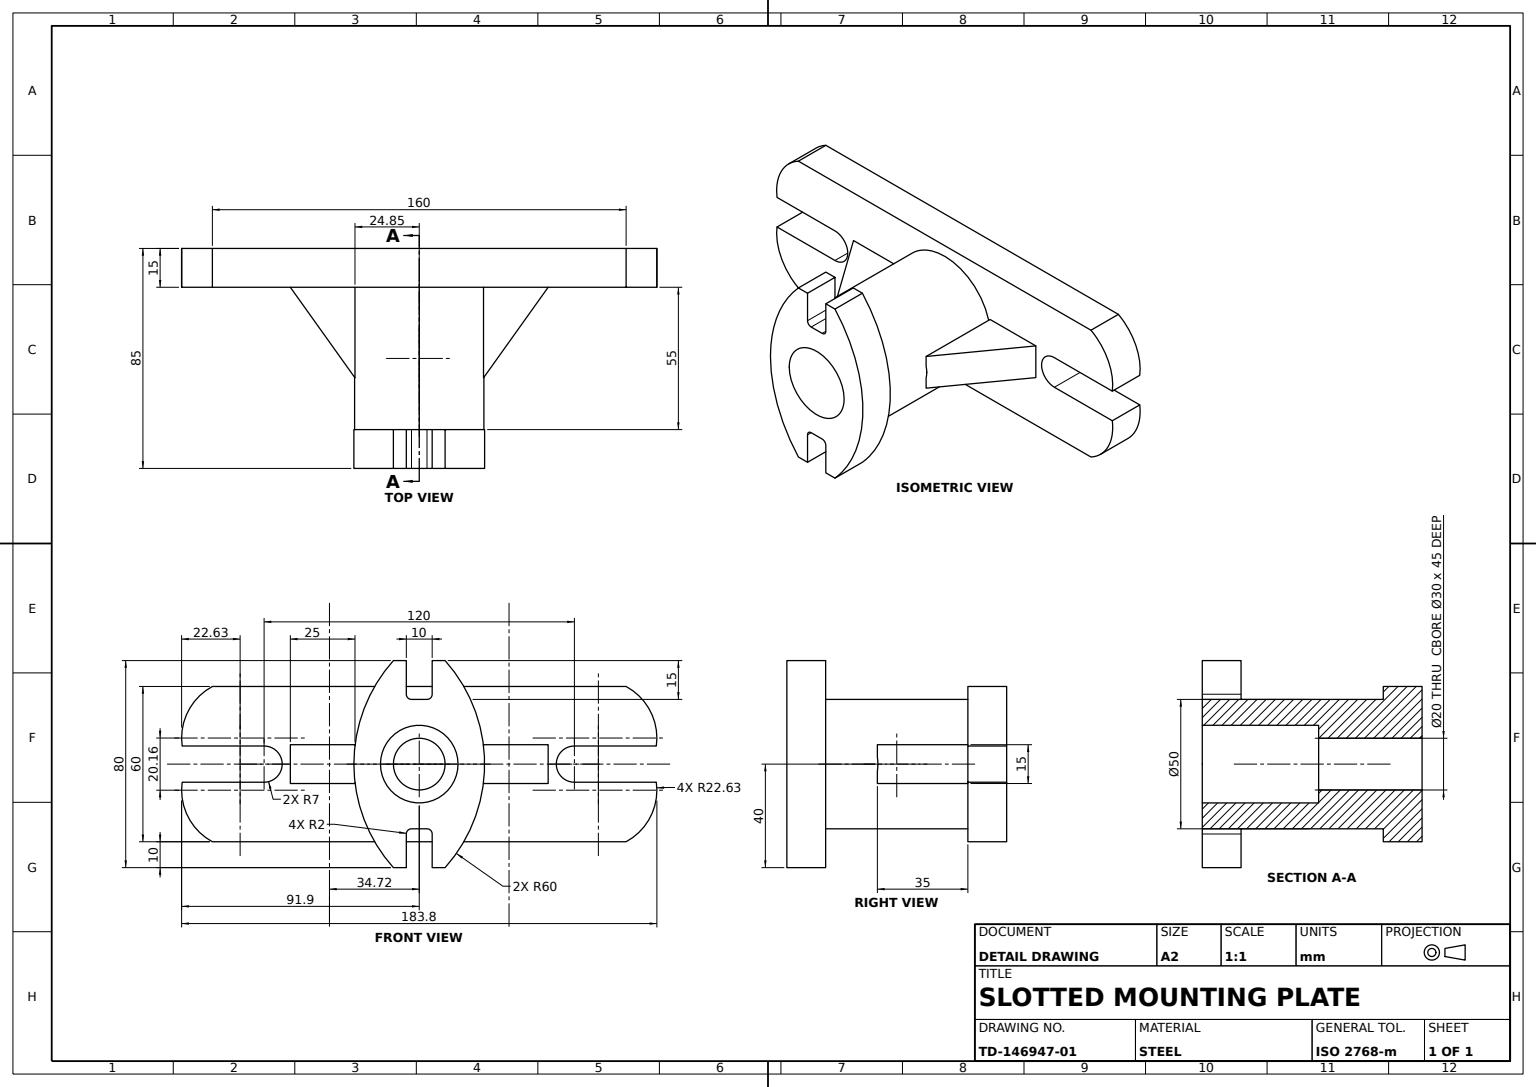
SolidWorks part; units mm, degrees
material "Plain Carbon Steel"
ref_plane "Front Plane" through (0, 0, 0) normal (0, 0, 1) x (1, 0, 0)
ref_plane "Top Plane" through (0, 0, 0) normal (0, 1, 0) x (1, 0, 0)
ref_plane "Right Plane" through (0, 0, 0) normal (1, 0, 0) x (0, 0, -1)
sketch "Flange Plate Sketch" plane through (0, 0, 0) normal (0, 0, 1) x (1, 0, 0)
  line L0 (0, 80.3458) -> (0, -81.9597) construction
  line L1 (-122.6513, 0) -> (117.3487, 0) construction
  line L3 (-80, 30) -> (80, 30)
  line L5 (-80, -30) -> (80, -30)
  line L7 (-80, 30) -> (80, -30) construction
  line L8 (-80, -30) -> (80, 30) construction
  line L14 (-60, -7) -> (-91.6879, -7)
  line L15 (-60, 7) -> (-91.6879, 7)
  line L16 (60, 7) -> (91.6879, 7)
  line L17 (60, -7) -> (91.6879, -7)
  arc A0 (-60, -7) -> (-60, 7) centre (-60, 0) ccw
  arc A1 (60, -7) -> (60, 7) centre (60, 0) cw
  arc A2 (-91.6879, -7) -> (-80, -30) centre (-69.2707, -10.078) ccw
  arc A3 (-91.6879, 7) -> (-80, 30) centre (-69.2707, 10.078) cw
  arc A4 (91.6879, 7) -> (80, 30) centre (69.2707, 10.078) ccw
  arc A5 (91.6879, -7) -> (80, -30) centre (69.2707, -10.078) cw
  point P5 (0, 0)
  dimension "D3" = 14
  dimension "D6" = 22.6275
  dimension "D1" = 160
  dimension "D2" = 60
  dimension "D4" = 70
  dimension "D5" = 120
extrude "Flange Plate" add sketch "Flange Plate Sketch" along normal mid plane 15
sketch "Hub Sketch" plane through (0, 0, 7.5) normal (0, 0, 1) x (1, 0, 0)
  circle A0 centre (0, 0) radius 25
  dimension "D1" = 50
extrude "Hub Ø50" add sketch "Hub Sketch" along normal blind 55
sketch "Hub Bore Sketch" plane through (0, 0, 62.5) normal (0, 0, 1) x (1, 0, 0)
  circle A0 centre (0, 0) radius 15
  dimension "D1" = 30
extrude "Hub Bore Ø30" cut sketch "Hub Bore Sketch" against normal through all
sketch "Slotted Collar Sketch" plane through (0, 0, 62.5) normal (0, 0, 1) x (1, 0, 0)
  line L0 (0, 44) -> (0, -44) construction
  line L1 (-104.0539, 0) -> (131.1722, 0) construction
  line L2 (5, -27) -> (5, -40)
  line L5 (-3, -25) -> (3, -25)
  line L6 (-5, 25) -> (5, 25)
  line L7 (-5, -27) -> (-5, -40)
  line L8 (-5, -40) -> (-10, -40)
  line L9 (5, -40) -> (10, -40)
  line L10 (5, 40) -> (10, 40)
  line L11 (-5, 40) -> (-10, 40)
  line L12 (-5, 27) -> (-5, 40)
  line L13 (-3, 25) -> (3, 25)
  line L14 (5, 27) -> (5, 40)
  arc A0 (10, 40) -> (10, -40) centre (-34.7214, 0) cw
  arc A1 (5, -27) -> (3, -25) centre (3, -27) ccw
  arc A2 (-5, -27) -> (-3, -25) centre (-3, -27) cw
  arc A3 (-5, 27) -> (-3, 25) centre (-3, 27) ccw
  arc A4 (5, 27) -> (3, 25) centre (3, 27) cw
  arc A5 (-10, 40) -> (-10, -40) centre (34.7214, 0) ccw
  circle A6 centre (0, 0) radius 15 construction
  point P5 (0, 25)
  point P6 (0, -25)
  point P8 (-5, -25)
  point P10 (5, -25)
  dimension "D3" = 2
  dimension "D6" = 60
  dimension "D1" = 88
  dimension "D2" = 10
  dimension "D4" = 5
  dimension "D5" = 13
  dimension "D7" = 34.7214
extrude "Slotted Collar" add sketch "Slotted Collar Sketch" along normal blind 15
ref_plane "Gusset Plane" through (0, 0, 0) normal (0, 1, 0) x (1, 0, 0)
sketch "Gusset Sketch" plane through (0, 0, 0) normal (0, 1, 0) x (1, 0, 0)
  line L0 (-24.8529, -7.5) -> (-24.8529, -42.5)
  line L1 (80, -7.5) -> (-80, -7.5) construction
  line L2 (-24.8529, -42.5) -> (-49.8529, -7.5)
  line L3 (-49.8529, -7.5) -> (-24.8529, -7.5)
  dimension "D1" = 25
  dimension "D2" = 35
  dimension "D3" = 24.8529
extrude "Gusset" add sketch "Gusset Sketch" along normal mid plane 15
mirror "Gusset Mirror" about plane through (0, 0, 0) normal (1, 0, 0) of "Gusset"
sketch "Collar Face Boss Sketch" plane through (0, 0, 77.5) normal (0, 0, 1) x (1, 0, 0)
  circle A0 centre (0, 0) radius 15 construction
  circle A1 centre (0, 0) radius 15
extrude "Collar Face Boss" add sketch "Collar Face Boss Sketch" against normal through all contours A1
sketch "Through Bore Ø20 Sketch" plane through (0, 0, 77.5) normal (0, 0, 1) x (1, 0, 0)
  circle A0 centre (0, 0) radius 10
  dimension "D1" = 20
extrude "Through Bore Ø20" cut sketch "Through Bore Ø20 Sketch" against normal through all
sketch "Collar Bore Ø30 Sketch" plane through (0, 0, 77.5) normal (0, 0, 1) x (1, 0, 0)
  circle A0 centre (0, 0) radius 15
  dimension "D1" = 30
extrude "Collar Bore Ø30 Depth 45" cut sketch "Collar Bore Ø30 Sketch" against normal blind 45
